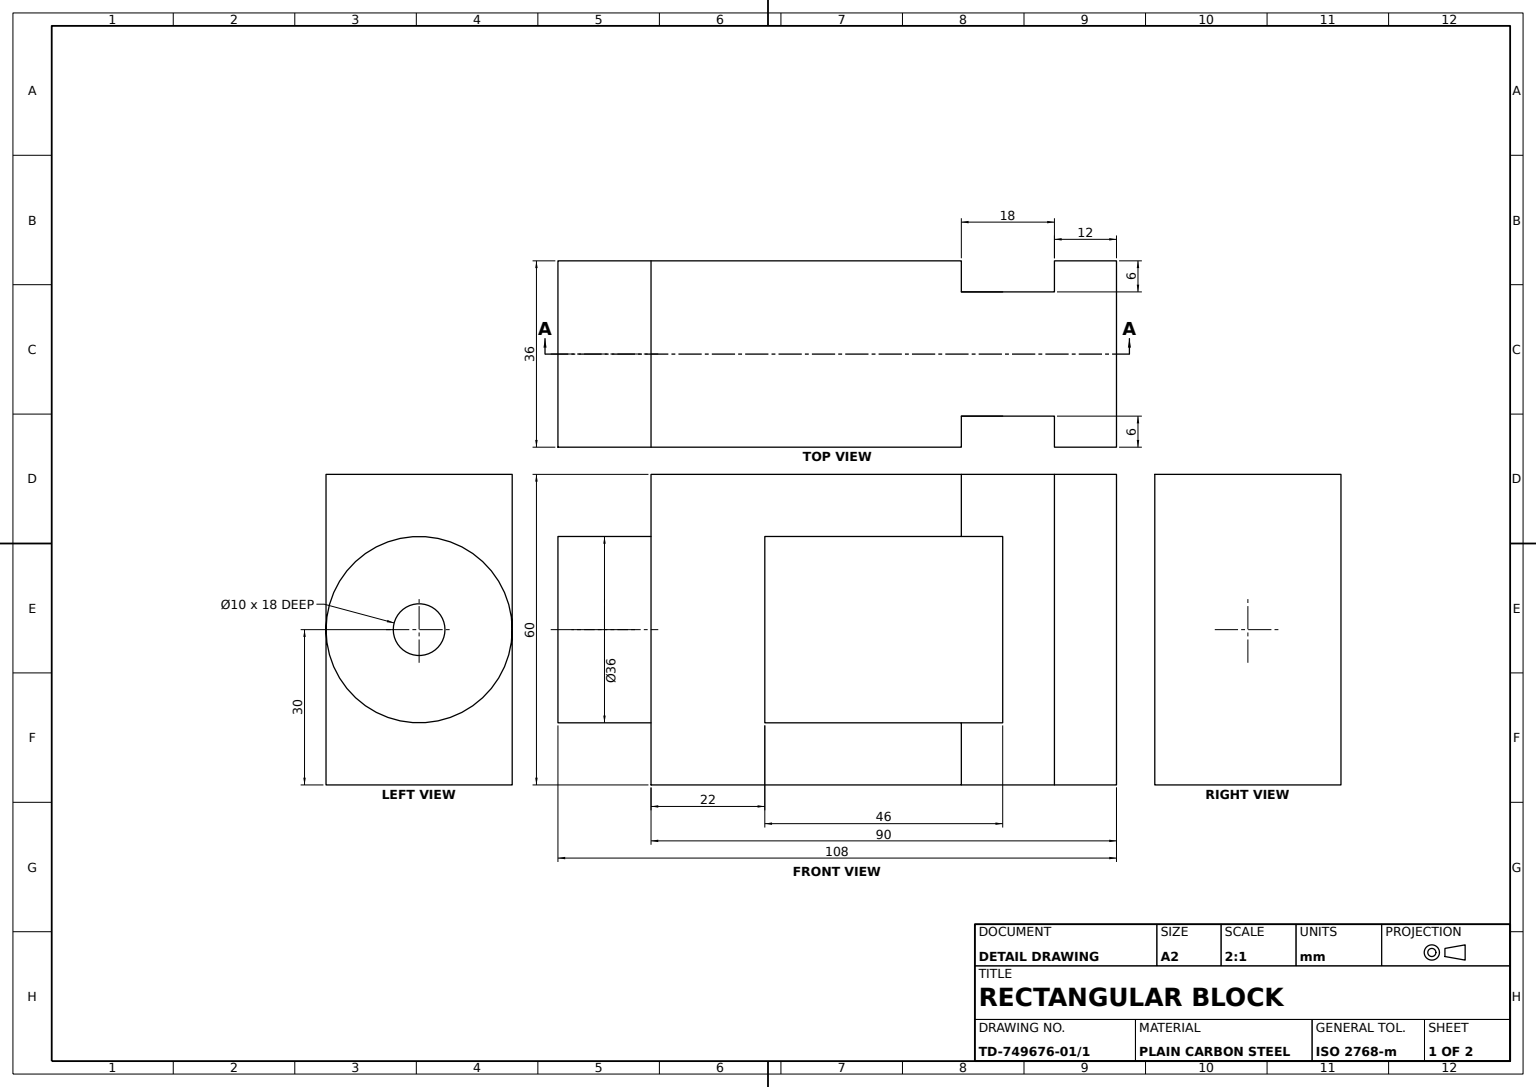
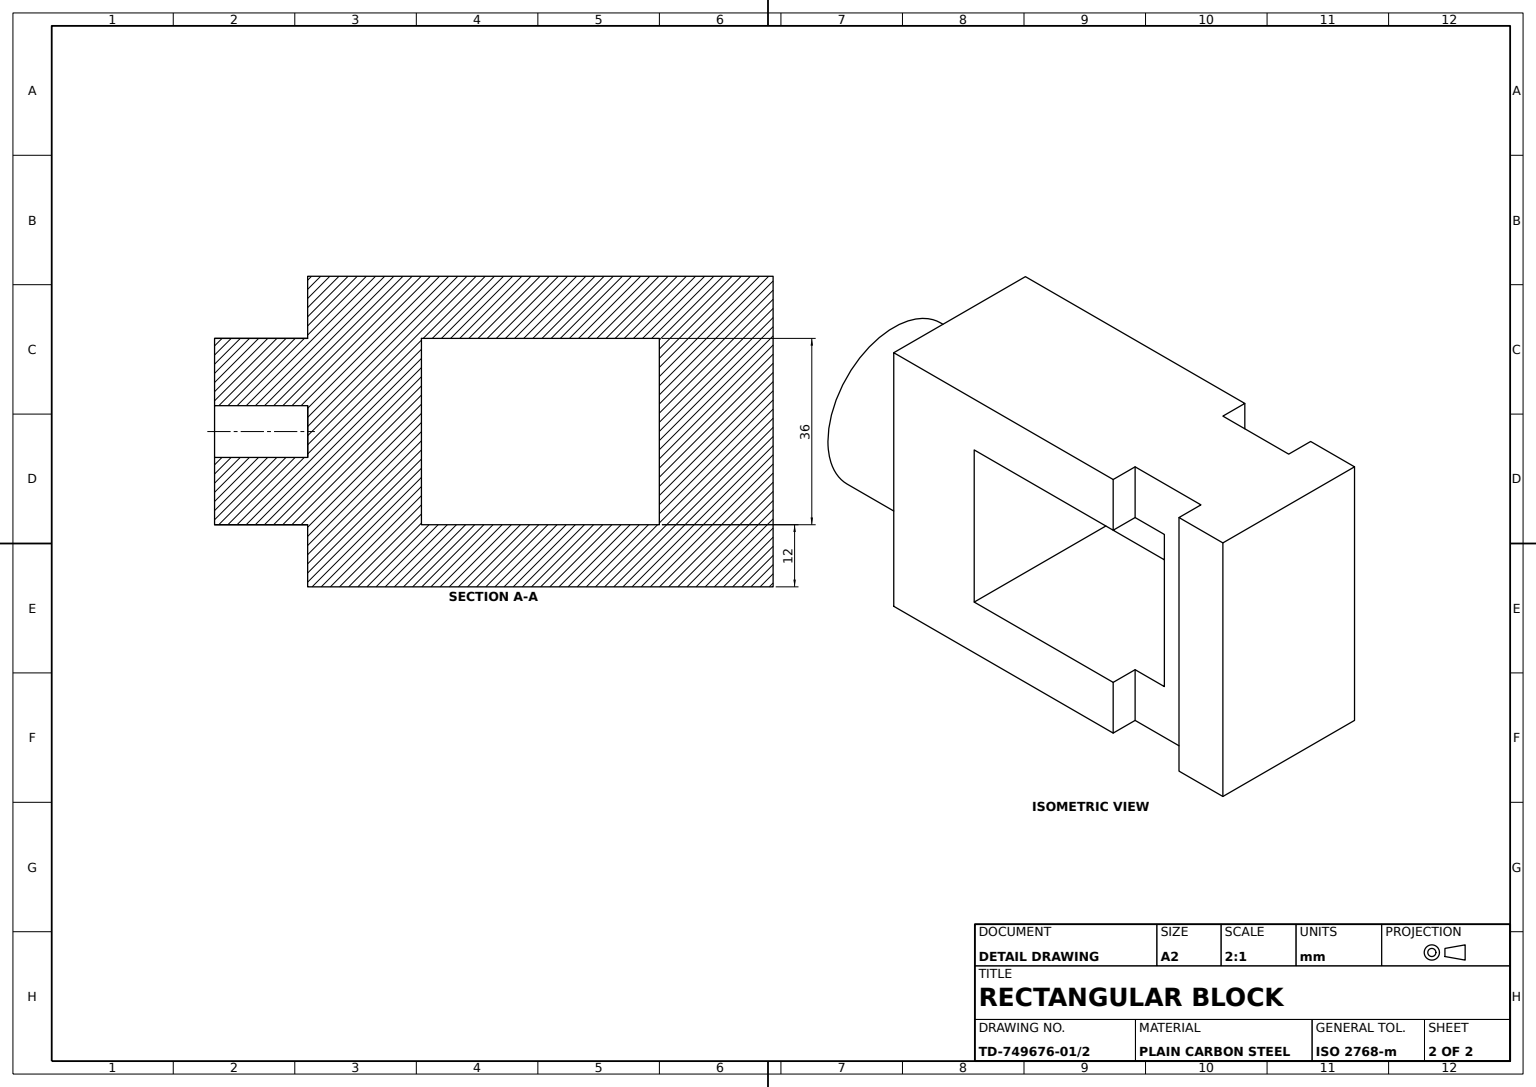
from build123d import *

# Parameters (mm, degrees)
BASE_BLOCK_SKETCH_W        = 90
BASE_BLOCK_SKETCH_H        = 60
BASE_BLOCK_DEPTH           = 36
WINDOW_SKETCH_W            = 46
WINDOW_SKETCH_H            = 36
THROUGH_WINDOW_46X36_DEPTH = 36
BOSS_SKETCH_R              = 18
CYLINDRICAL_BOSS_DEPTH     = 18
BOSS_BORE_SKETCH_R         = 5
BOSS_BORE_DEPTH            = 18
TOP_NOTCHES_SKETCH_W       = 18
TOP_NOTCHES_SKETCH_H       = 6
TOP_NOTCHES_DEPTH          = 95.154128959
END_NOTCH_SKETCH_W         = 18
END_NOTCH_SKETCH_H         = 6
END_NOTCH_DEPTH            = 95.154128959


with BuildPart() as part:
    # Base Block Sketch → Base Block (new body)
    with BuildSketch(Plane.XY):
        Rectangle(BASE_BLOCK_SKETCH_W, BASE_BLOCK_SKETCH_H)
    extrude(amount=BASE_BLOCK_DEPTH)

    # Window Sketch → Through Window 46x36 (cut)
    with BuildSketch(Plane.XY.offset(36)):
        Rectangle(WINDOW_SKETCH_W, WINDOW_SKETCH_H)
    extrude(amount=-THROUGH_WINDOW_46X36_DEPTH, mode=Mode.SUBTRACT)

    # Boss Sketch → Cylindrical Boss (add)
    with BuildSketch(Plane.ZY.offset(45)):
        with Locations((18, 0)):
            Circle(BOSS_SKETCH_R)
    extrude(amount=CYLINDRICAL_BOSS_DEPTH)

    # Boss Bore Sketch → Boss Bore (cut)
    with BuildSketch(Plane.ZY.offset(63)):
        with Locations((18, 0)):
            Circle(BOSS_BORE_SKETCH_R)
    extrude(amount=-BOSS_BORE_DEPTH, mode=Mode.SUBTRACT)

    # Top Notches Sketch → Top Notches (cut, through all)
    with BuildSketch(Plane.XZ.offset(30)):
        with Locations((24, 3)):
            Rectangle(TOP_NOTCHES_SKETCH_W, TOP_NOTCHES_SKETCH_H)
    extrude(amount=-TOP_NOTCHES_DEPTH, mode=Mode.SUBTRACT)

    # End Notch Sketch → End Notch (cut, through all)
    with BuildSketch(Plane.XZ.offset(30)):
        with Locations((24, 33)):
            Rectangle(END_NOTCH_SKETCH_W, END_NOTCH_SKETCH_H)
    extrude(amount=-END_NOTCH_DEPTH, mode=Mode.SUBTRACT)


solid = part.part
